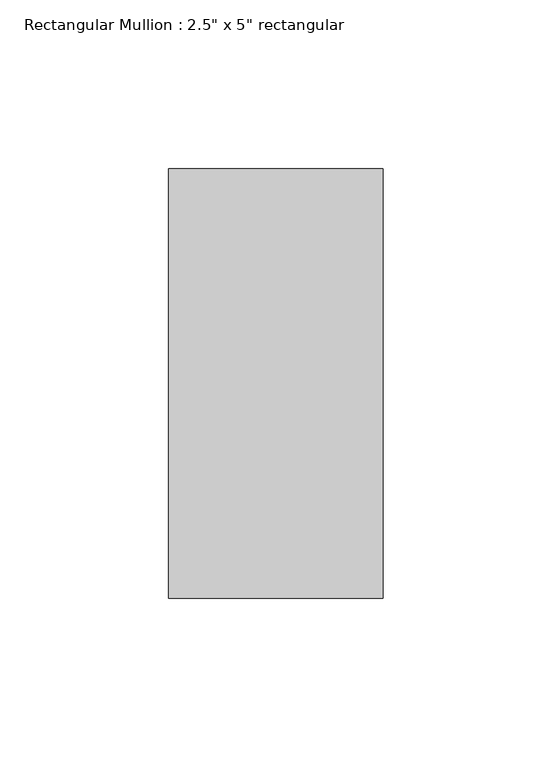
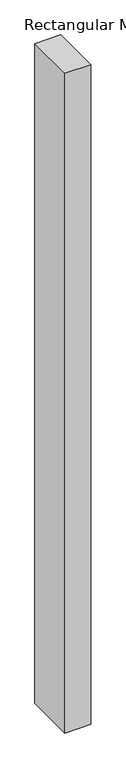
"""IFC4 building model written with IfcOpenShell, lengths in millimetres: member geometry."""

from ifc_helpers import new_model, si_unit, frame, origin, place, context, project, spatial, polyline, outline, extrude, source, transform, mapped, element, save


def member_cba59155(model_context):
    return source(origin(), model_context, "Body", "SweptSolid", [
        extrude(outline(polyline([(31.75, 63.5), (31.75, -63.5), (-31.75, -63.5), (-31.75, 63.5), (31.75, 63.5)])), frame((0.0, 0.0, -1701.8), z_axis=(0.0, 0.0, 1.0), x_axis=(1.0, 0.0, 0.0)), (0.0, 0.0, 1.0), 1701.8),
    ])


if __name__ == "__main__":
    model = new_model("IFC4")
    model_context = context("Model", 3, world=origin())
    ifc_project = project(units=[si_unit("LENGTHUNIT", "METRE", prefix="MILLI")], contexts=[model_context])
    site = spatial("IfcSite", under=ifc_project)
    building = spatial("IfcBuilding", under=site)
    placement = place(None, origin())
    member_shape = member_cba59155(model_context)
    element("IfcMember", 1, ObjectType="Rectangular Mullion : 2.5\" x 5\" rectangular", at=placement, inside=building, context=model_context, shape_type="MappedRepresentation", body=[
        mapped(member_shape, transform((0.0, 0.0, 0.0), x_axis=(1.0, 0.0, 0.0), y_axis=(0.0, 1.0, 0.0), z_axis=(0.0, 0.0, 1.0))),
    ])
    save(model, "model.ifc")

# Revit data of these elements
# Type "Rectangular Mullion : 2.5\" x 5\" rectangular"
#   built-in parameter 1007304 = 0.416667 (stored number, unit not read)
#   built-in parameter 1007301 = 0.104167 (stored number, unit not read)
#   built-in parameter 1007300 = 0.104167 (stored number, unit not read)
# Element 1 (IfcMember, "Rectangular Mullion : 2.5\" x 5\" rectangular")
#   Materials on its faces: "Aluminum"
# Materials
#   "Aluminum": class "Metal", colour RGB 247 247 247, transparency 0, Description = "Aluminum 6061", Cost = 0
